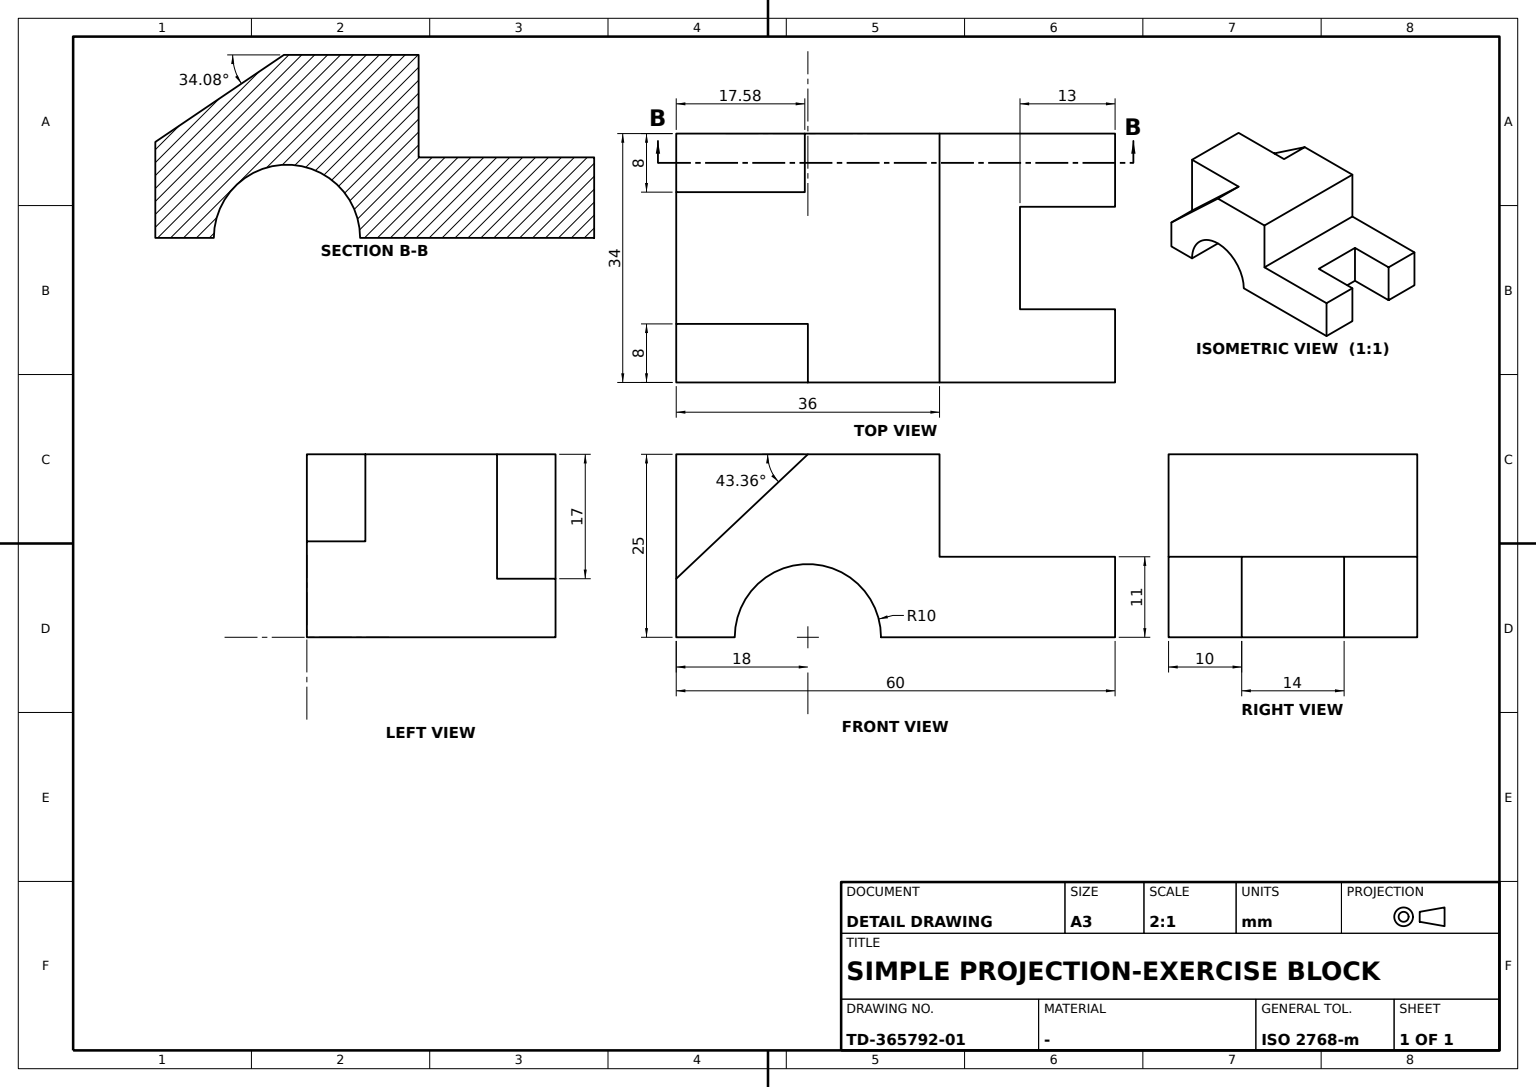
CATIA V5 part; units mm, degrees
sketch "Sketch1" plane through (0, 0, 0) normal (1, 0, 0) x (0, 1, 0)
  point P0 (-18, 0)
  line L0 (-18, 0) -> (-10, 0)
  arc A0 (10, 0) -> (-10, 0) centre (0, 0) ccw
  point P1 (10, 0)
  line L1 (10, 0) -> (42, 0)
  line L2 (42, 0) -> (42, 11)
  line L3 (42, 11) -> (18, 11)
  line L4 (18, 11) -> (18, 25)
  line L5 (18, 25) -> (-18, 25)
  line L6 (-18, 25) -> (-18, 0)
  dimension "length L5" = 36
  dimension "length L6" = 25
  dimension "length L2" = 11
  dimension "radius A0" = 10
  dimension "distance L6 L2" = 60
  dimension "length L0" = 8
  constraint coincidence P0 x-axis
  constraint coincidence P1 x-axis
  constraint horizontal L0 x-axis
  constraint horizontal L1 x-axis
  constraint horizontal L3 x-axis
  constraint horizontal L5 x-axis
  constraint vertical L2 y-axis
  constraint vertical L4 y-axis
  constraint vertical L6 y-axis
extrude "Pad1" add sketch "Sketch1" along normal mid plane 34
sketch "Sketch2" plane through (17, 0, 0) normal (1, 0, 0) x (0, 1, 0)
  line L0 (-18, 8) -> (0, 25)
  point P0 (-18, 8)
  point P1 (0, 25)
  line L1 (-18, 25) -> (-18, 0) construction
  line L2 (-18, 25) -> (-18, 8)
  point P2 (-18, 25)
  point P3 (-18, 0)
  line L3 (18, 25) -> (-18, 25) construction
  line L4 (0, 25) -> (-18, 25)
  point P4 (-18, 25)
  dimension "distance P1 P2" = 18
  dimension "distance P0 P3" = 8
  constraint coincidence P1 L3
  constraint coincidence P0 L1
  constraint coincidence P2 P4
extrude "Pocket1" cut sketch "Sketch2" against normal blind 8
sketch "Sketch3" plane through (-17, 0, 0) normal (-1, 0, 0) x (0, -1, 0)
  line L0 (0.4201, 25) -> (18, 13.1052)
  point P0 (0.0022, 25.2827)
  point P1 (25.5453, 8)
  line L1 (18, 25) -> (18, 13.1052)
  point P2 (18, 25)
  point P3 (18, 0)
  line L2 (-18, 25) -> (18, 25) construction
  line L3 (0.4201, 25) -> (18, 25)
  point P4 (18, 25)
  point P5 (0.4201, 25)
  point P6 (0.4201, 25)
  dimension "distance P1 P3 y axis" = 8
  dimension "distance P0 P2" = 18
  constraint coincidence L0 P5
  constraint coincidence L2 P6
  constraint coincidence P2 P4
  constraint coincidence P5 P6
extrude "Pocket2" cut sketch "Sketch3" against normal blind 8
sketch "Sketch4" plane through (0, 0, 11) normal (0, 0, 1) x (1, 0, 0)
  point P0 (0, 35.5)
  line L0 (7, 42) -> (7, 29)
  line L1 (7, 29) -> (-7, 29)
  line L2 (-7, 29) -> (-7, 42)
  line L3 (-7, 42) -> (7, 42)
  line L4 (-17, 42) -> (17, 42) construction
  dimension "length L0" = 13
  dimension "length L3" = 14
  constraint coincidence P0 y-axis
  constraint coincidence L3 L4
  constraint vertical L0 y-axis
  constraint vertical L2 y-axis
  constraint horizontal L1 x-axis
  constraint horizontal L3 x-axis
  constraint equidistance L0 L2 P0
  constraint equidistance L1 L3 P0
extrude "Pocket3" cut sketch "Sketch4" against normal blind 13
